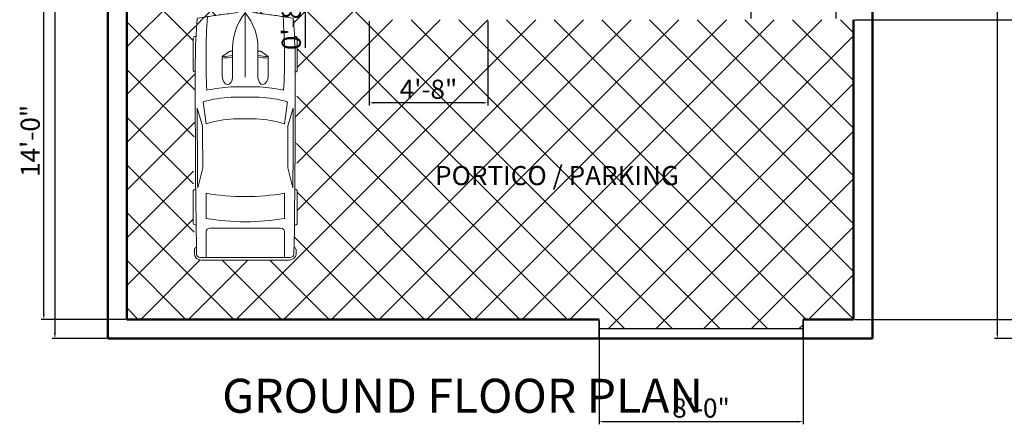
# Model space of a CAD drawing. Units: inches. Extents: x 3587 to 4539, y 1613 to 2440.
# Tile 1 of 8: x 3603 to 4067, y 1613 to 1803. Entities that reach past the tile are written whole.
import ezdxf

# ---------------------------------------------------------------- set-up
doc = ezdxf.new("R2010")
doc.units = ezdxf.units.IN
for name, color, linetype, lineweight in [('A-ANNO-DIMS', 2, 'Continuous', 18), ('A-ANNO-TITL', 7, 'Continuous', 35), ('A-AREA-IDEN', 7, 'Continuous', 25), ('A-DOOR', 3, 'Continuous', 25), ('A-FLOR-PATT', 252, 'Continuous', 13), ('A-SITE-VEHI', 9, 'Continuous', 13), ('A-WALL', 7, 'Continuous', 50)]:
    doc.layers.add(name, color=color, linetype=linetype, lineweight=lineweight)
doc.styles.get("Standard").update_dxf_attribs({"font": 'arial.ttf'})
doc.dimstyles.new('ISO-25', dxfattribs={"dimtxt": 9, "dimasz": 2.5, "dimexe": 1.25, "dimexo": 0.625, "dimtad": 1, "dimlunit": 3, "dimtxsty": 'Standard', "dimcen": 2.5, "dimadec": 0, "dimazin": 0, "dimtfac": 1, "dimtmove": 0, "dimatfit": 3, "dimfxl": 1, "dimarcsym": 0})

# ---------------------------------------------------------------- blocks, each defined once
blk = doc.blocks.new('*U6')
for p, q in [((21.10406751471477, 37.40863046792069), (21.10406751471477, 36.83230215753705)), ((46.55368679439944, 38.88847654282876), (22.35054758993934, 38.88847654282876)), ((47.80016686962392, 37.39011648242055), (47.80016686962392, 37.40863046792069)), ((135.4513231603356, 37.07354110333037), (135.4513231603356, 37.40863046792069)), ((136.6978032355602, 38.88847654282876), (160.90094244002, 38.88847654282867)), ((162.1474225152445, 37.40863046792049), (162.1474225152445, 36.77402019194128)), ((70.0302824853563, 31.53613089391356), (86.40615155322342, 29.35124891408057)), ((87.98532186932616, 31.87120872459877), (74.75900729854769, 35.92175679182955)), ((134.313356548143, 35.6043097713567), (119.2882629232503, 31.77757799177584)), ((186.4728846989705, -33.49860931502491), (186.4728846989718, 33.49860931502465)), ((188.3990091454065, -32.75868627757393), (188.3990091454077, 32.75868627757058)), ((138.4228833961707, 29.35124891408074), (157.2465674415997, 29.35124891408074)), ((164.515393597658, 26.39155676426461), (164.5153935976578, -26.39155676426503)), ((186.4728846989718, 29.35124891408083), (167.0083537481071, 29.35124891408083)), ((32.26591480791686, 11.62530558863241), (36.12873726252356, 17.16961494239206)), ((36.12873726252356, 17.16961494239206), (50.93891189819171, 17.16961494239206)), ((29.77279020470884, 9.505833383620029), (51.68362801571248, 9.505833383620029)), ((32.12291633764599, 9.505833383620029), (32.12291633764599, 11.15369945057711)), ((58.9167604809788, -10.77488335095668), (58.9167604809788, 10.77488335095617)), ((66.55009204259746, -10.5288681329018), (66.55009204259746, 10.52886813290129)), ((82.73706193978568, 8.496039918672748), (82.73706193978568, -8.49603991867258)), ((186.4728846989718, -10.5288681329018), (186.4728846989718, 10.52886813290129)), ((3.266462181856987, 6.128290093440767), (0.1022408397004821, 0.4060708604429806)), ((-4.43e-14, -2.558e-13), (51.68362801571248, -2.558e-13)), ((0.1022408397004821, -0.4060708604432933), (3.266462181856987, -6.128290093441194)), ((29.77279020470884, -9.50583338362054), (51.68362801571248, -9.50583338362054)), ((32.12291633764599, -9.50583338362054), (32.12291633764599, -11.15369945057762)), ((32.26591480791686, -11.62530558863292), (36.12873726252356, -17.16961494239257)), ((36.12873726252356, -17.16961494239257), (50.93891189819171, -17.16961494239257)), ((86.40615155322318, -29.35124891408145), (70.03028248535594, -31.53613089391442)), ((157.2465674415997, -29.35124891408117), (138.4228833961707, -29.35124891408126)), ((167.008353748107, -29.35124891408126), (186.4728846989707, -29.35124891408108)), ((21.10406751471477, -37.4086304679212), (21.10406751471477, -36.83230215753756)), ((87.98532186932607, -31.87120872459903), (74.7590072985476, -35.92175679182964)), ((134.3133565481428, -35.60430977135721), (119.2882629232503, -31.77757799177618)), ((162.1474225152445, -37.408630467921), (162.1474225152445, -36.77402019194179)), ((46.55368679439944, -38.88847654282927), (22.35054758993934, -38.88847654282927)), ((47.80016686962392, -37.39011648242107), (47.80016686962392, -37.4086304679212)), ((135.4513231603355, -37.07354110333088), (135.4513231603355, -37.4086304679212)), ((136.6978032355602, -38.88847654282927), (160.9009424400199, -38.88847654282918))]:
    blk.add_line(p, q)
for centre, major_axis, ratio, start_param, end_param in [((41.19115208863305, -490.8631038926156), (1.294e-13, 528.2339998381949), 0.8423038695439741, 0.0028100083536837, 0.0755983031096952), ((22.35054758993934, 37.40863046792072), (2.08e-14, -1.479846074908118), 0.842303869543976, 3.141592653589776, 4.712388980384677), ((64.48199294511879, -10555.61767587835), (1.907644e-10, 10593.02630634627), 0.842303869543847, -0.0133969486112073, 0.0027970409639888), ((46.55368679439944, 37.40863046792072), (2.2e-14, 1.479846074908118), 0.8423038695439758, -1.570796326794884, 1.73e-14), ((136.6978032355602, 37.40863046792072), (2.357e-13, -1.479846074908118), 0.842303869543976, 3.141592653589603, 4.712388980384554), ((160.90094244002, 37.40863046792052), (5.59e-14, 1.479846074908118), 0.842303869543976, -1.570796326794865, 4.44e-14), ((180.6280394947615, 35.8381667808375), (7.4e-14, 2.219769112362114), 0.8423038695439693, -0.0130174256259048, 1.249894140392862), ((64.48199294754608, -10556.35759891604), (1.349839377e-06, 10595.3130398087), 0.8423038681351469, -0.0133969484821159, -0.0130174254969711), ((183.9799245485216, 32.75868627756583), (8.56e-14, -5.246425615115243), 0.8423038695439737, 1.570796326795794, 3.128195704978164), ((266.0300214172791, -27.52442688366631), (1.966072e-10, 313.3077612809058), 0.8423038695435284, 1.367075990158062, 1.391760499156098), ((37.47375371777758, -593.9621830607928), (6.21e-14, -623.32820996736), 0.8423038695439826, 3.09604606856106, 3.200911180495224), ((135.2911776514449, 5.387441675478555), (2.2715e-12, 81.77258453065997), 0.8423038695439563, 1.245306111696802, 1.507880129813836), ((64.4819929449925, -10555.61767590795), (1.9177683e-09, -10591.54646030096), 0.8423038695482963, 3.133765086725325, 3.140440689641252), ((95.78879860270445, -3666.353346297651), (1.949864e-10, -3698.236159209632), 0.8423038695446962, 3.134048706297306, 3.14409775411291), ((183.9799245485226, 33.49860931502124), (3e-16, -2.959692149816168), 0.8423038695439952, 1.570796326796048, 3.128195704978389), ((259.1750197310735, -27.52442688366614), (1.506617e-10, -305.3028914627677), 0.8423038695443789, 4.528606069860317, 4.561837674556238), ((134.4003789125686, 5.387441675477674), (4.276e-13, -89.7774543484738), 0.84230386954398, 4.44948196380473, 4.652344057257214), ((149.595361812917, 2.799442537139299), (8.561e-13, -79.57966406425402), 0.842303869543983, 4.372215489277867, 4.640744122441986), ((17.08207736189386, -1.421e-13), (6.87e-14, 147.0179238898305), 0.8423038695439764, 4.511394369635731, 4.913383591133647), ((35.90576140732288, -1.421e-13), (6.87e-14, 147.0179238898305), 0.8423038695439764, 4.511394369635731, 4.913383591133647), ((167.0083537481071, 26.39155676426464), (1.394e-13, 2.959692149816236), 0.842303869543976, 5.55e-14, 1.57079632679492), ((-204.4946649195746, 52.39684969293512), (4.12053e-11, -250.9602162198571), 0.8423038695441164, 1.385369446298923, 1.434372047871027), ((13.03653510440275, 17.00972444508943), (1.2303e-12, 27.41599049210566), 0.8423038695439277, 4.435146050259648, 4.718221029521873), ((14.20086229321332, 17.00972444508943), (1.2303e-12, 27.41599049210566), 0.8423038695439277, 4.435146050259648, 4.718221029521873), ((50.7902773840875, 13.33772416300607), (6.340077547122382, -0.356608581037027), 0.6038335755719145, -1.39555193967809, 1.581314658479915), ((29.77279020470884, -46.66302566589627), (5.12e-14, 56.16885904951626), 0.842303869543976, 7e-16, 0.5903187773915901), ((32.74615637525823, 11.15369945057713), (1.313e-13, 0.7399230374541176), 0.8423038695439091, 0.8797135699495516, 1.570796326795045), ((0.6232400376122422, -1.421e-13), (1e-16, -0.7399230374541245), 0.842303869543842, 4.131459131953847, 5.293318828815531), ((-204.4946649195746, -52.39684969293552), (4.02945e-11, 250.9602162198562), 0.8423038695441192, -1.43437204787103, -1.385369446298926), ((29.77279020470884, 46.66302566589578), (4.004e-13, 56.16885904951626), 0.8423038695439734, 2.55127387619821, 3.141592653589801), ((32.74615637525823, -11.1536994505777), (1.3e-13, -0.7399230374541176), 0.8423038695439093, 4.712388980384541, 5.403471737230034), ((13.03653510440275, -17.00972444508983), (1.2568e-12, -27.41599049210552), 0.8423038695439318, 1.564964277657711, 1.848039256919935), ((14.20086229321332, -17.00972444508983), (1.2568e-12, -27.41599049210552), 0.8423038695439318, 1.564964277657711, 1.848039256919935), ((134.4003789125684, -5.387441675478584), (4.2949e-12, -89.77745434847827), 0.8423038695439354, -1.510751403667474, -1.307889310215002), ((135.2911776514465, -5.387441675480715), (3.2038e-12, -81.77258453066244), 0.8423038695439492, -1.50788012981387, -1.245306111696839), ((149.5953618129329, -2.799442537137565), (4.0897e-12, -79.57966406427697), 0.8423038695439419, -1.499151468852248, -1.230622835688196), ((259.1750197310694, 27.52442688365929), (1.08535e-11, 305.3028914629043), 0.8423038695439974, 1.721347632622872, 1.754579237318777), ((266.0300214172791, 27.52442688366566), (8.75241e-11, 313.3077612806533), 0.8423038695441819, 1.749832154434603, 1.774516663432659), ((37.47375371777847, 593.9621830607904), (1.1693e-12, -623.3282099673584), 0.8423038695439528, -0.0593185269054384, 0.0455465850287298), ((167.008353748107, -26.39155676426503), (1.02e-14, -2.959692149816192), 0.8423038695439885, 4.712388980384686, 6.283185307179581), ((41.19115208863322, 490.8631038926152), (1.37757e-11, -528.2339998381949), 0.8423038695440652, -0.0755983031097181, -0.0028100083537155), ((64.48199294495228, 10555.61767590795), (6.117947e-10, 10593.02630637587), 0.8423038695458146, 3.138795612625926, 3.154989602201039), ((64.48199294503607, 10555.61767590793), (1.6049794e-09, -10591.54646030094), 0.8423038695397146, 0.0011519639481523, 0.0078275668641468), ((95.78879860271888, 3666.35334629765), (1.637818e-10, -3698.236159209629), 0.8423038695447546, -0.0025051005232382, 0.007543947292366), ((180.6280394947581, -35.83816678083949), (2.274e-13, -2.219769112363032), 0.8423038695439803, -1.249894138785958, 0.0130174256254374), ((183.9799245485216, -33.4986093150211), (9.3e-15, 2.959692149816141), 0.8423038695439732, 3.154989602201626, 4.71238898038339), ((183.9799245485177, -32.7586862775633), (2.428e-13, -5.246425615118353), 0.8423038695439808, 0.0133969486110846, 1.570796326792831), ((22.35054758993934, -37.40863046792117), (2.2e-14, 1.479846074908118), 0.8423038695439758, 1.570796326794908, 3.14159265358981), ((46.55368679439944, -37.40863046792117), (2.08e-14, -1.479846074908118), 0.842303869543976, -1.69e-14, 1.570796326794884), ((136.6978032355602, -37.40863046792109), (1.56e-14, -1.479846074908162), 0.8423038695440105, -1.570796326794875, -1.27e-14), ((160.9009424400199, -37.408630467921), (1.969e-13, 1.479846074908162), 0.8423038695440109, 3.141592653589951, 4.712388980384771), ((64.48199294197605, 10556.3575989598), (9.365289701e-07, 10595.31303985772), 0.8423038705260315, 3.154610079306566, 3.154989602290631)]:
    blk.add_ellipse(centre, major_axis=major_axis, ratio=ratio, start_param=start_param, end_param=end_param)
at = {"extrusion": (0, 0, -1)}
blk.add_ellipse((50.7902773840875, -13.33772416300655), major_axis=(6.340077547122382, 0.3566085810370246), ratio=0.6038335755719145, start_param=-1.39555193967809, end_param=1.581314658479915, dxfattribs=at)
blk = doc.blocks.new('*D14')
at = {"layer": 'A-ANNO-DIMS', "color": 0, "lineweight": -2, "transparency": 16777216}
for p, q in [((3643.898273186453, 2372.933027064171), (3618.38722522892, 2372.933027064171)), ((3619.63722522892, 2370.433027064171), (3619.63722522892, 1655.43302706417)), ((3643.898273186453, 1652.93302706417), (3618.38722522892, 1652.93302706417))]:
    blk.add_line(p, q, dxfattribs=at)
at = {"layer": 'A-ANNO-DIMS', "color": 0, "transparency": 16777216}
for points in [[(3619.220558562253, 2370.433027064171), (3620.053891895587, 2370.433027064171), (3619.63722522892, 2372.933027064171)], [(3619.220558562253, 1655.43302706417), (3620.053891895587, 1655.43302706417), (3619.63722522892, 1652.93302706417)]]:
    blk.add_solid(points, dxfattribs=at)
at = {"layer": 'Defpoints', "color": 0, "transparency": 16777216}
for p in [(3644.523273186453, 2372.933027064171), (3619.63722522892, 1652.93302706417), (3644.523273186453, 1652.93302706417)]:
    blk.add_point(p, dxfattribs=at)
at = {"layer": 'A-ANNO-DIMS', "color": 0, "transparency": 16777216, "insert": (3614.417068339424, 2019.45310680197), "char_height": 9, "attachment_point": 5, "rotation": 90}
blk.add_mtext("60'", dxfattribs=at)
blk = doc.blocks.new('*D28')
at = {"layer": 'A-ANNO-DIMS', "color": 0, "lineweight": -2, "transparency": 16777216}
for p, q in [((4087.490632697894, 2372.933027064171), (4061.979584740361, 2372.933027064171)), ((4063.229584740361, 2370.433027064171), (4063.229584740361, 1655.43302706417)), ((4087.490632697894, 1652.93302706417), (4061.979584740361, 1652.93302706417))]:
    blk.add_line(p, q, dxfattribs=at)
at = {"layer": 'A-ANNO-DIMS', "color": 0, "transparency": 16777216}
for points in [[(4062.812918073695, 2370.433027064171), (4063.646251407027, 2370.433027064171), (4063.229584740361, 2372.933027064171)], [(4062.812918073695, 1655.43302706417), (4063.646251407027, 1655.43302706417), (4063.229584740361, 1652.93302706417)]]:
    blk.add_solid(points, dxfattribs=at)
at = {"layer": 'Defpoints', "color": 0, "transparency": 16777216}
for p in [(4088.115632697895, 2372.933027064171), (4063.229584740361, 1652.93302706417), (4088.115632697895, 1652.93302706417)]:
    blk.add_point(p, dxfattribs=at)
at = {"layer": 'A-ANNO-DIMS', "color": 0, "transparency": 16777216, "insert": (4058.009427850866, 2019.45310680197), "char_height": 9, "attachment_point": 5, "rotation": 90}
blk.add_mtext("60'", dxfattribs=at)
blk = doc.blocks.new('*D73')
at = {"layer": 'A-ANNO-DIMS', "color": 0, "lineweight": -2, "transparency": 16777216}
for p, q in [((3738.545915569897, 1846.866674009694), (3736.1209155699, 1846.866674009694)), ((3737.3709155699, 1844.366674009694), (3737.3709155699, 1840.867390120344)), ((3738.545915569897, 1838.367390120344), (3736.1209155699, 1838.367390120344)), ((3737.3709155699, 1838.367390120344), (3737.3709155699, 1789.721755741081))]:
    blk.add_line(p, q, dxfattribs=at)
at = {"layer": 'A-ANNO-DIMS', "color": 0, "transparency": 16777216}
for points in [[(3736.954248903233, 1844.366674009694), (3737.787582236567, 1844.366674009694), (3737.3709155699, 1846.866674009694)], [(3736.954248903233, 1840.867390120344), (3737.787582236567, 1840.867390120344), (3737.3709155699, 1838.367390120344)]]:
    blk.add_solid(points, dxfattribs=at)
at = {"layer": 'Defpoints', "color": 0, "transparency": 16777216}
for p in [(3739.170915569898, 1846.866674009694), (3737.3709155699, 1838.367390120344), (3739.170915569898, 1838.367390120344)]:
    blk.add_point(p, dxfattribs=at)
at = {"layer": 'A-ANNO-DIMS', "color": 0, "transparency": 16777216, "insert": (3732.092436715876, 1812.794572930711), "char_height": 9, "attachment_point": 5, "rotation": 90}
blk.add_mtext('0\'-8 1/2"', dxfattribs=at)
blk = doc.blocks.new('*D80')
at = {"layer": 'A-ANNO-DIMS', "color": 0, "lineweight": -2, "transparency": 16777216}
for p, q in [((3996.148273000001, 1802.933027000001), (4095.873273000004, 1802.933027000001)), ((4094.623273000004, 1664.433027000001), (4094.623273000004, 1800.433027000001)), ((3996.148273000001, 1661.933027000001), (4095.873273000004, 1661.933027000001))]:
    blk.add_line(p, q, dxfattribs=at)
at = {"layer": 'A-ANNO-DIMS', "color": 0, "transparency": 16777216}
for points in [[(4094.206606333337, 1800.433027000001), (4095.03993966667, 1800.433027000001), (4094.623273000004, 1802.933027000001)], [(4094.206606333337, 1664.433027000001), (4095.03993966667, 1664.433027000001), (4094.623273000004, 1661.933027000001)]]:
    blk.add_solid(points, dxfattribs=at)
at = {"layer": 'Defpoints', "color": 0, "transparency": 16777216}
for p in [(3995.523273000002, 1802.933027000001), (4094.623273000004, 1802.933027000001), (3995.523273000002, 1661.933027000001)]:
    blk.add_point(p, dxfattribs=at)
at = {"layer": 'A-ANNO-DIMS', "color": 0, "transparency": 16777216, "insert": (4089.403116110508, 1732.433026999999), "char_height": 9, "attachment_point": 5, "rotation": 90}
blk.add_mtext('11\'-9"', dxfattribs=at)
blk = doc.blocks.new('*D83')
at = {"layer": 'A-ANNO-DIMS', "color": 0, "lineweight": -2, "transparency": 16777216}
for p, q in [((3875.779602, 1661.308027), (3875.779602, 1612.583027)), ((3971.779602, 1661.308027), (3971.779602, 1612.583027)), ((3878.279602, 1613.833027), (3969.279602, 1613.833027))]:
    blk.add_line(p, q, dxfattribs=at)
at = {"layer": 'A-ANNO-DIMS', "color": 0, "transparency": 16777216}
for points in [[(3878.279602, 1614.249693666667), (3878.279602, 1613.416360333333), (3875.779602, 1613.833027)], [(3969.279602, 1614.249693666667), (3969.279602, 1613.416360333333), (3971.779602, 1613.833027)]]:
    blk.add_solid(points, dxfattribs=at)
at = {"layer": 'Defpoints', "color": 0, "transparency": 16777216}
for p in [(3875.779602, 1661.933027), (3971.779602, 1661.933027), (3971.779602, 1613.833027)]:
    blk.add_point(p, dxfattribs=at)
at = {"layer": 'A-ANNO-DIMS', "color": 0, "transparency": 16777216, "insert": (3923.779602000001, 1619.053183889495), "char_height": 9, "attachment_point": 5}
blk.add_mtext('8\'-0"', dxfattribs=at)
blk = doc.blocks.new('*D89')
at = {"layer": 'A-ANNO-DIMS', "color": 0, "lineweight": -2, "transparency": 16777216}
for p, q in [((3947.419563, 1803.558027), (3947.419563, 1843.283027)), ((3949.919563, 1842.033027), (3984.919563, 1842.033027)), ((3987.419563, 1803.558027), (3987.419563, 1843.283027))]:
    blk.add_line(p, q, dxfattribs=at)
at = {"layer": 'A-ANNO-DIMS', "color": 0, "transparency": 16777216}
for points in [[(3949.919563, 1842.449693666667), (3949.919563, 1841.616360333333), (3947.419563, 1842.033027)], [(3984.919563, 1842.449693666667), (3984.919563, 1841.616360333333), (3987.419563, 1842.033027)]]:
    blk.add_solid(points, dxfattribs=at)
at = {"layer": 'Defpoints', "color": 0, "transparency": 16777216}
for p in [(3987.419563, 1842.033027), (3947.419563, 1802.933027), (3987.419563, 1802.933027)]:
    blk.add_point(p, dxfattribs=at)
at = {"layer": 'A-ANNO-DIMS', "color": 0, "transparency": 16777216, "insert": (3967.419563, 1847.256253466575), "char_height": 9, "attachment_point": 5}
blk.add_mtext('3\'-4"', dxfattribs=at)
blk = doc.blocks.new('*D93')
at = {"layer": 'A-ANNO-DIMS', "color": 0, "lineweight": -2, "transparency": 16777216}
for p, q in [((3767.523273, 1802.308027), (3767.523273, 1762.583026999999)), ((3823.451685, 1802.308027), (3823.451685, 1762.583026999999)), ((3820.951685, 1763.833027), (3770.023273, 1763.833027))]:
    blk.add_line(p, q, dxfattribs=at)
at = {"layer": 'A-ANNO-DIMS', "color": 0, "transparency": 16777216}
for points in [[(3770.023273, 1764.249693666666), (3770.023273, 1763.416360333333), (3767.523273, 1763.833027)], [(3820.951685, 1764.249693666666), (3820.951685, 1763.416360333333), (3823.451685, 1763.833027)]]:
    blk.add_solid(points, dxfattribs=at)
at = {"layer": 'Defpoints', "color": 0, "transparency": 16777216}
for p in [(3767.523273, 1802.933027), (3823.451685, 1802.933027), (3767.523273, 1763.833027)]:
    blk.add_point(p, dxfattribs=at)
at = {"layer": 'A-ANNO-DIMS', "color": 0, "transparency": 16777216, "insert": (3795.487479, 1769.053183889495), "char_height": 9, "attachment_point": 5}
blk.add_mtext('4\'-8"', dxfattribs=at)
blk = doc.blocks.new('*D94')
at = {"layer": 'A-ANNO-DIMS', "color": 0, "lineweight": -2, "transparency": 16777216}
for p, q in [((3652.898273000002, 1829.933027000001), (3613.173273000004, 1829.933027000001)), ((3614.423273000003, 1664.433027000001), (3614.423273000003, 1827.433027000001)), ((3652.898273000002, 1661.933027000001), (3613.173273000004, 1661.933027000001))]:
    blk.add_line(p, q, dxfattribs=at)
at = {"layer": 'A-ANNO-DIMS', "color": 0, "transparency": 16777216}
for points in [[(3614.006606333337, 1827.433027000001), (3614.839939666671, 1827.433027000001), (3614.423273000003, 1829.933027000001)], [(3614.006606333337, 1664.433027000001), (3614.839939666671, 1664.433027000001), (3614.423273000003, 1661.933027000001)]]:
    blk.add_solid(points, dxfattribs=at)
at = {"layer": 'Defpoints', "color": 0, "transparency": 16777216}
for p in [(3614.423273000003, 1829.933027000001), (3653.523273000002, 1829.933027000001), (3653.523273000002, 1661.933027000001)]:
    blk.add_point(p, dxfattribs=at)
at = {"layer": 'A-ANNO-DIMS', "color": 0, "transparency": 16777216, "insert": (3609.203116110508, 1745.933026999999), "char_height": 9, "attachment_point": 5, "rotation": 90}
blk.add_mtext('14\'-0"', dxfattribs=at)

msp = doc.modelspace()

# ---------------------------------------------------------------- hatches: boundary and pattern name
at = {"layer": 'A-FLOR-PATT'}
h = msp.add_hatch(dxfattribs=at)
h.set_pattern_fill('ANSI37', color=256, scale=5)
h.set_pattern_definition([(45, (0, 0), (-11.22532015133644, 11.22532015133644), []), (135, (0, 0), (-11.22532015133644, -11.22532015133644), [])])
h.paths.add_polyline_path([(3995.523273186451, 1802.933027064169), (3767.523273186451, 1802.933027064169), (3767.523273186451, 1829.93302706417), (3653.523273186451, 1829.933027064169), (3653.523273186451, 1661.93302706417), (3773.523273186451, 1661.933027064169), (3875.779602316032, 1661.93302706417), (3875.779602316032, 1657.433027064169), (3971.779602316032, 1657.433027064169), (3971.779602316032, 1661.933027064169), (3995.523273186451, 1661.933027064169)])
edge = h.paths.add_edge_path(flags=16)
edge.add_ellipse((-2931.215124755575, 1767.796697431512), major_axis=(-6663.991736021397, 5.49378e-10), ratio=0.8423038695427154, start_angle=179.6161332212123, end_angle=180.0902290885991, ccw=False)
edge.add_ellipse((3732.776611265823, 1722.366284151288), major_axis=(0.9309598341942544, 1.21e-13), ratio=0.8423038695440663, start_angle=-7.503331289626658e-12, end_angle=89.99999999999261, ccw=False)
edge.add_line((3733.707571100018, 1722.825629213573), (3733.707571100018, 1706.680929544622))
edge.add_ellipse((3732.776611265823, 1707.140274606908), major_axis=(-0.9309598341942548, 1.2281e-12), ratio=0.8423038695440661, start_angle=90.00000000007549, end_angle=180.0000000000756, ccw=False)
edge.add_ellipse((-2931.215124755575, 1767.796697431512), major_axis=(-6663.991736021397, 5.49378e-10), ratio=0.8423038695427154, start_angle=179.3813568036855, end_angle=179.4717285281868, ccw=False)
edge.add_ellipse((3731.78864458569, 1694.730108904805), major_axis=(1.396439751291259, 5.988e-13), ratio=0.8423038695438281, start_angle=-0.6282372162187926, end_angle=68.4647566009865, ccw=False)
edge.add_ellipse((-2931.680604672821, 1767.796697429986), major_axis=(-6665.430302531707, 1.2246408655e-06), ratio=0.8423038675137327, start_angle=179.3534459134782, end_angle=179.3717627943114, ccw=False)
edge.add_ellipse((3729.85136698139, 1692.621463683659), major_axis=(-3.300486181350725, 3.344e-13), ratio=0.8423038695438854, start_angle=90.0000000000714, end_angle=179.3534459029256, ccw=False)
edge.add_line((3729.851366981394, 1689.841451401731), (3688.634889588928, 1689.841451401732))
edge.add_ellipse((3688.634889588934, 1692.621463683661), major_axis=(-3.300486181352529, 1.172e-12), ratio=0.8423038695439762, start_angle=0.6465540970764891, end_angle=89.99999999988921, ccw=False)
edge.add_ellipse((10350.16686127067, 1767.796697433487), major_axis=(-6665.430302568726, 2.939407166e-06), ratio=0.842303874418981, start_angle=0.6282372415100781, end_angle=0.6465541223432183, ccw=False)
edge.add_ellipse((3686.697611984631, 1694.730108904807), major_axis=(-1.396439751291707, 7.567e-13), ratio=0.8423038695440721, start_angle=-68.46475649595652, end_angle=0.6282372162064007, ccw=False)
edge.add_ellipse((10349.70138134452, 1767.796697431614), major_axis=(-6663.991736040017, 4.813117e-10), ratio=0.8423038695453691, start_angle=0.5282714718214834, end_angle=0.6465540970651205, ccw=False)
edge.add_ellipse((3685.7096453045, 1707.140274606908), major_axis=(-0.9309598341942544, 1.7437e-12), ratio=0.8423038695440663, start_angle=1.0732037480920553e-10, end_angle=90.00000000010732, ccw=False)
edge.add_line((3684.778685470305, 1706.680929544623), (3684.778685470305, 1722.825629213573))
edge.add_ellipse((3685.7096453045, 1722.366284151288), major_axis=(-0.9309598341942548, 1.208e-13), ratio=0.8423038695440661, start_angle=-89.9999999999925, end_angle=7.503331289626658e-12, ccw=False)
edge.add_ellipse((10349.70138134452, 1767.796697431614), major_axis=(-6663.991736040017, 4.813117e-10), ratio=0.8423038695453691, start_angle=-0.09022908858901246, end_angle=0.38386677879640274, ccw=False)
edge.add_line((3685.721292311014, 1778.291106478928), (3685.164301659653, 1778.291106478928))
edge.add_ellipse((3685.7096453045, 1779.07525754966), major_axis=(0.9309598341942544, 1.21e-13), ratio=0.8423038695440663, start_angle=179.9999999999926, end_angle=269.99999999999255, ccw=False)
edge.add_line((3684.778685470305, 1779.07525754966), (3684.778685470305, 1794.760612156325))
edge.add_ellipse((3685.7096453045, 1794.30126709404), major_axis=(-0.9309598341942544, 9.038e-13), ratio=0.8423038695438219, start_angle=-89.99999999994441, end_angle=5.559286364587024e-11, ccw=False)
edge.add_ellipse((4018.041348289437, 1782.448787070864), major_axis=(-332.3079644858751, 4.99005e-11), ratio=0.842303869543478, start_angle=-3.6504275856905224, end_angle=-2.1799503136365956, ccw=False)
edge.add_ellipse((3726.558534476647, 1641.004376020469), major_axis=(-197.0995135497352, 6.041863e-10), ratio=0.8423038695462189, start_angle=-77.87403444754023, end_angle=-76.2194710103264, ccw=False)
edge.add_ellipse((3726.558534476642, 1645.316805090899), major_axis=(192.0637112431616, 1.152005e-10), ratio=0.8423038695435717, start_angle=100.20953899710878, end_angle=102.44462729340961, ccw=False)
edge.add_ellipse((3676.280671358373, 1937.007853276476), major_axis=(-157.877150362268, 8.51952e-11), ratio=0.8423038695445018, start_angle=99.25656600723244, end_angle=102.554932644168)
edge.add_line((3705.38786791314, 1806.306919092921), (3709.243128285161, 1808.438766310234))
edge.add_line((3709.243128285161, 1808.438766310234), (3713.098388657182, 1806.306919092921))
edge.add_ellipse((3742.20558521195, 1937.007853276476), major_axis=(157.8771503623125, 4.39696e-11), ratio=0.8423038695442709, start_angle=257.4450673558467, end_angle=260.7434339927823)
edge.add_ellipse((3691.927722093676, 1645.316805090896), major_axis=(192.0637112426421, 4.323641e-10), ratio=0.8423038695457922, start_angle=77.55537270642571, end_angle=79.79046100272637, ccw=False)
edge.add_ellipse((3691.927722093676, 1641.004376020469), major_axis=(197.0995135501296, 1.621172e-10), ratio=0.8423038695445964, start_angle=76.21947101045492, end_angle=77.87403444766869, ccw=False)
edge.add_ellipse((3400.444908280885, 1782.448787070864), major_axis=(-332.3079644858756, 3.24129e-11), ratio=0.8423038695443688, start_angle=182.1799503136508, end_angle=183.6504275857046, ccw=False)
edge.add_ellipse((3732.776611265823, 1794.30126709404), major_axis=(0.9309598341942544, 9.038e-13), ratio=0.8423038695438222, start_angle=-5.559286364587024e-11, end_angle=89.99999999994441, ccw=False)
edge.add_line((3733.707571100018, 1794.760612156325), (3733.707571100018, 1778.615912487374))
edge.add_ellipse((3732.776611265823, 1779.07525754966), major_axis=(-0.9309598341942548, 1.2281e-12), ratio=0.8423038695440661, start_angle=90.00000000007549, end_angle=180.0000000000756, ccw=False)
edge = h.paths.add_edge_path(flags=0)
edge.add_ellipse((-2931.215124774197, 1767.796697431592), major_axis=(6663.060776205826, 1.8394224e-09), ratio=0.8423038695493525, start_angle=-0.3777641939256, end_angle=-0.05559431351520061, ccw=False)
edge.add_line((3731.641526931722, 1723.866321304078), (3729.234159271377, 1733.318492652809))
edge.add_ellipse((1402.768312261676, 1748.10182571592), major_axis=(2326.532049492193, 1.008783e-10), ratio=0.8423038695441537, start_angle=-0.3640763488928343, end_angle=0.1208973690301654)
edge.add_line((3729.293061648444, 1753.010933175826), (3731.841230421537, 1761.331506395292))
edge = h.paths.add_edge_path(flags=0)
edge.add_line((3729.08226675093, 1764.306310966309), (3727.707774227574, 1754.004377129606))
edge.add_ellipse((3711.004236149284, 1714.252528809921), major_axis=(-50.06295730256603, 1.815e-12), ratio=0.8423038695439442, start_angle=247.2080851224121, end_angle=265.1299304028664)
edge.add_line((3714.587921941819, 1756.312573310335), (3703.898334628504, 1756.312573310335))
edge.add_ellipse((3707.48202042104, 1714.252528809911), major_axis=(50.06295730257607, 2.3708e-12), ratio=0.8423038695439807, start_angle=94.87006959713298, end_angle=112.7919148775837)
edge.add_line((3690.778482342749, 1754.004377129606), (3689.403989819393, 1764.30631096631))
edge.add_ellipse((3705.853929980028, 1723.25118153539), major_axis=(-51.44250677627033, 5.286e-13), ratio=0.8423038695439773, start_angle=-85.72257903694498, end_angle=-68.16504620329079, ccw=False)
edge.add_line((3702.61949796478, 1766.49567212521), (3715.866758605543, 1766.49567212521))
edge.add_ellipse((3712.632326590294, 1723.251181535391), major_axis=(-51.4425067762775, 8.5929e-12), ratio=0.8423038695438458, start_angle=248.1650462032994, end_angle=265.7225790369539, ccw=False)
edge = h.paths.add_edge_path(flags=0)
edge.add_ellipse((3717.633788426009, 1776.410050850261), major_axis=(0.2243397276943869, 3.988494237425664), ratio=0.6038335755718559, start_angle=106.34259195430289, end_angle=270.9979857249751, ccw=False)
edge.add_line((3715.223175278389, 1775.848050808502), (3715.223175278389, 1789.63199109895))
edge.add_ellipse((3679.88777614854, 1789.631991098951), major_axis=(-35.33539912984816, 5.5728e-12), ratio=0.8423038695440471, start_angle=180.0000000000086, end_angle=209.4385695979881)
edge.add_ellipse((3738.598480421783, 1789.631991098951), major_axis=(35.33539912984861, 3.5956e-12), ratio=0.842303869543988, start_angle=150.5614304020151, end_angle=179.9999999999942)
edge.add_line((3703.263081291934, 1789.631991098951), (3703.263081291934, 1775.848050808502))
edge.add_ellipse((3700.852468144314, 1776.410050850261), major_axis=(-0.2243397276943869, 3.988494237425664), ratio=0.6038335755718559, start_angle=89.00201427502492, end_angle=253.6574080456972, ccw=False)
edge.add_line((3698.441854996694, 1776.316546015567), (3698.441854996694, 1785.633513473865))
edge.add_line((3698.441854996694, 1785.633513473865), (3702.058856064699, 1788.15354474419))
edge.add_line((3702.058856064699, 1788.15354474419), (3703.263081291934, 1788.15354474419))
edge.add_line((3703.263081291934, 1788.15354474419), (3703.263081291934, 1789.631991098951))
edge.add_ellipse((3738.598480421783, 1789.631991098951), major_axis=(35.33539912984861, 3.5956e-12), ratio=0.842303869543988, start_angle=150.5614304020151, end_angle=179.9999999999942, ccw=False)
edge.add_ellipse((3679.88777614854, 1789.631991098951), major_axis=(-35.33539912984816, 5.5728e-12), ratio=0.8423038695440471, start_angle=180.0000000000087, end_angle=209.4385695979881, ccw=False)
edge.add_line((3715.223175278389, 1789.631991098951), (3715.223175278389, 1788.15354474419))
edge.add_line((3715.223175278389, 1788.15354474419), (3716.427400505623, 1788.15354474419))
edge.add_line((3716.427400505623, 1788.15354474419), (3720.044401573629, 1785.633513473865))
edge.add_line((3720.044401573629, 1785.633513473865), (3720.044401573629, 1776.316546015567))
edge = h.paths.add_edge_path(flags=0)
edge.add_line((3727.707774227574, 1721.281049431593), (3727.707774227574, 1709.439213936003))
edge.add_ellipse((3709.243128285161, 1785.773785876993), major_axis=(92.48785016817327, 5.807e-13), ratio=0.8423038695439611, start_angle=256.4018653097688, end_angle=283.59813469023004, ccw=False)
edge.add_line((3690.778482342749, 1709.439213936003), (3690.778482342749, 1721.281049431593))
edge.add_ellipse((3709.243128285161, 1797.615621372584), major_axis=(92.48785016817327, 5.807e-13), ratio=0.8423038695439611, start_angle=256.4018653097688, end_angle=283.59813469023)
edge = h.paths.add_edge_path(flags=0)
edge.add_line((3727.707774227574, 1703.298148918879), (3727.707774227574, 1691.053161542195))
edge.add_line((3727.707774227574, 1691.053161542195), (3690.778482342749, 1691.053161542196))
edge.add_line((3690.778482342749, 1691.053161542196), (3690.778482342749, 1703.298148918879))
edge.add_ellipse((3692.640402011137, 1703.298148918879), major_axis=(1.861919668388509, 8.39e-13), ratio=0.8423038695439441, start_angle=89.9999999999742, end_angle=179.9999999999742, ccw=False)
edge.add_line((3692.640402011137, 1704.866451060343), (3725.845854559185, 1704.866451060343))
edge.add_ellipse((3725.845854559185, 1703.298148918879), major_axis=(1.861919668388508, 1.025e-12), ratio=0.8423038695439441, start_angle=-3.149125404888764e-11, end_angle=89.99999999996851, ccw=False)
edge = h.paths.add_edge_path(flags=0)
edge.add_ellipse((6015.717944308645, 1748.10182571591), major_axis=(2326.532049492191, 7.14324e-11), ratio=0.8423038695472079, start_angle=179.8791026309652, end_angle=180.3640763488883)
edge.add_line((3689.252097298946, 1733.318492652807), (3686.844729638601, 1723.86632130408))
edge.add_ellipse((10349.70138134451, 1767.796697431562), major_axis=(6663.060776205814, 1.4769457e-09), ratio=0.8423038695377512, start_angle=180.0555943134864, end_angle=180.3777641938969, ccw=False)
edge.add_line((3686.645026148788, 1761.331506395283), (3689.19319492188, 1753.010933175827))
h.paths.add_polyline_path([(3795.361201859856, 1720.01661730307), (3924.209769390551, 1720.01661730307), (3924.209769390551, 1738.563002023398), (3795.361201859856, 1738.563002023398)], flags=24)

# ---------------------------------------------------------------- linework, layer by layer
at = {"layer": 'A-DOOR'}
for p, q in [((3875.779602316032, 1652.933027064169), (3875.779602316032, 1661.933027064169)), ((3971.779602316032, 1652.933027064169), (3971.779602316032, 1661.933027064169)), ((3971.779602316032, 1657.433027064169), (3875.779602316032, 1657.433027064169))]:
    msp.add_line(p, q, dxfattribs=at)
at = {"layer": 'A-WALL'}
for p, q in [((3644.523273186451, 2372.933027064169), (3644.523273186451, 1652.933027064169)), ((4004.523273186451, 2372.933027064169), (4004.523273186451, 1652.933027064169)), ((3653.523273186451, 1829.93302706417), (3653.523273186451, 1661.933027064169)), ((3995.523273186451, 1802.93302706417), (3995.523273186451, 1661.933027064169)), ((3773.523273186451, 1661.933027064169), (3653.523273186451, 1661.93302706417)), ((3875.779602316033, 1661.93302706417), (3773.523273186451, 1661.93302706417)), ((3995.523273186451, 1661.933027064169), (3971.779602316032, 1661.933027064169)), ((4004.523273186451, 1652.933027064169), (3644.523273186451, 1652.933027064169))]:
    msp.add_line(p, q, dxfattribs=at)

# ---------------------------------------------------------------- block references
at = {"layer": 'A-SITE-VEHI', "xscale": 0.6290923427641268, "yscale": 0.6290923427641268, "zscale": 0.6290923427641268, "rotation": 270}
msp.add_blockref('*U6', (3709.243128285161, 1808.361825439456), dxfattribs=at)

# ---------------------------------------------------------------- texts
at = {"layer": 'A-ANNO-TITL', "insert": (3698.385285154262, 1633.999949119919), "char_height": 16, "attachment_point": 1}
msp.add_mtext_dynamic_manual_height_columns('GROUND FLOOR PLAN', width=307.5297505560302, gutter_width=12.5, heights=[0], dxfattribs=at)
at = {"layer": 'A-AREA-IDEN', "insert": (3798.581188217291, 1734.090628217123), "char_height": 9, "attachment_point": 1}
msp.add_mtext_dynamic_manual_height_columns('PORTICO / PARKING', width=162.4166489375966, gutter_width=12.5, heights=[0], dxfattribs=at)

# ---------------------------------------------------------------- dimensions: what is measured, and where the dimension line sits
at = {"layer": 'A-ANNO-DIMS'}
for base, p1, p2, picture, middle in [((3619.63722522892, 1652.93302706417), (3644.523273186451, 2372.933027064169), (3644.523273186451, 1652.933027064169), '*D14', (3619.637225228919, 2019.45310680197)), ((4063.229584740361, 1652.93302706417), (4088.115632697892, 2372.933027064169), (4088.115632697892, 1652.933027064169), '*D28', (4063.229584740361, 2019.45310680197))]:
    dim = msp.add_linear_dim(base=base, p1=p1, p2=p2, angle=90, dimstyle='ISO-25', override={"dimclrd": 0, "dimclre": 0, "dimclrt": 0}, dxfattribs=at)
    dim.commit()
    dim.dimension.update_dxf_attribs({"geometry": picture, "text_midpoint": middle, "dimtype": 160})
for base, p1, p2, picture, middle in [((3987.419563, 1842.033027), (3947.419563, 1802.933027), (3987.419563, 1802.933027), '*D89', (3967.419563, 1847.256253466575)), ((3971.779602, 1613.833027), (3875.779602, 1661.933027), (3971.779602, 1661.933027), '*D83', (3923.779602000001, 1619.053183889495))]:
    dim = msp.add_linear_dim(base=base, p1=p1, p2=p2, dimstyle='ISO-25', override={"dimdec": 1, "dimlfac": 1, "dimrnd": 0, "dimzin": 1, "dimdsep": 46, "dimlunit": 4, "dimfrac": 2}, dxfattribs=at)
    dim.commit()
    dim.dimension.update_dxf_attribs({"geometry": picture, "text_midpoint": middle})
for base, p1, p2, angle, picture, middle in [((3737.3709155699, 1838.367390120344), (3739.170915569896, 1846.866674009693), (3739.170915569896, 1838.367390120343), 270, '*D73', (3732.092436715876, 1812.794572930711)), ((3614.423273000003, 1829.933027000001), (3653.523273, 1661.933027), (3653.523273, 1829.933027), 90, '*D94', (3609.203116110508, 1745.933026999999)), ((3767.523273, 1763.833027), (3823.451685, 1802.933027), (3767.523273, 1802.933027), 180, '*D93', (3795.487479, 1769.053183889495)), ((4094.623273000004, 1802.933027000001), (3995.523273, 1661.933027), (3995.523273, 1802.933027), 90, '*D80', (4089.403116110508, 1732.433026999999))]:
    dim = msp.add_linear_dim(base=base, p1=p1, p2=p2, angle=angle, dimstyle='ISO-25', override={"dimdec": 1, "dimlfac": 1, "dimrnd": 0, "dimzin": 1, "dimdsep": 46, "dimlunit": 4, "dimfrac": 2}, dxfattribs=at)
    dim.commit()
    dim.dimension.update_dxf_attribs({"geometry": picture, "text_midpoint": middle})

doc.saveas('drawing.dxf')
